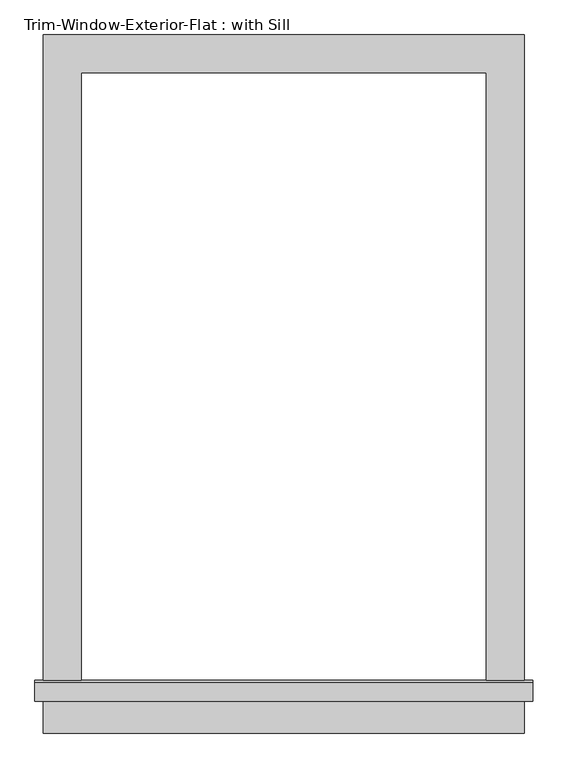
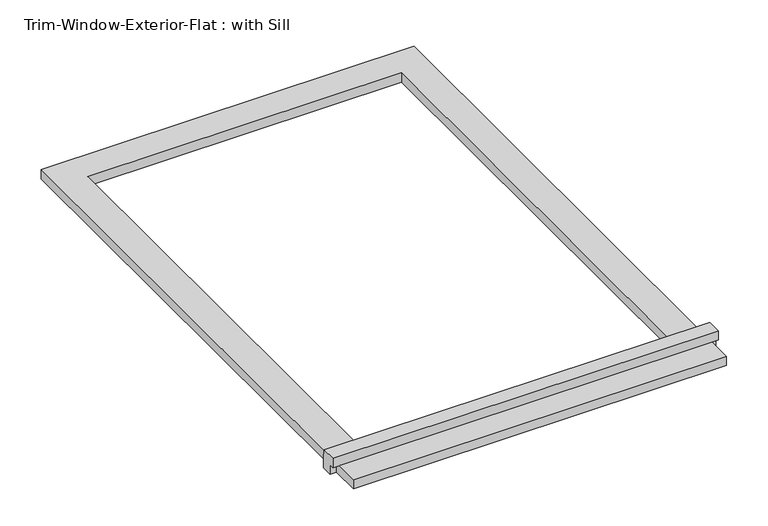
"""IFC4 building model written with IfcOpenShell, lengths in millimetres: proxy geometry, Trim-Window-Exterior-Flat : with Sill."""

from ifc_helpers import new_model, si_unit, frame, origin, origin_with_axes, place, context, project, spatial, polyline, outline, extrude, source, transform, mapped, element, save


def trim_window_exterior_flat_with_sill_a665a915(model_context):
    return source(origin(), model_context, "Body", "SweptSolid", [
        extrude(outline(polyline([(361.95, -936.5823709), (361.95, -993.7323709), (-361.95, -993.7323709), (-361.95, -936.5823709), (361.95, -936.5823709)])), origin_with_axes(), (0.0, 0.0, 1.0), 19.05),
        extrude(outline(polyline([(-946.15, 38.1), (-916.8580645, 38.1), (-914.4, 19.05), (-914.4, 0.0), (-936.5823709, 0.0), (-936.5823709, 19.05), (-946.15, 19.05), (-946.15, 38.1)])), frame((-374.65, 0.0, 0.0), z_axis=(1.0, 0.0, 0.0), x_axis=(0.0, 1.0, 0.0)), (0.0, 0.0, 1.0), 749.3),
        extrude(outline(polyline([(-361.95, 57.15), (361.95, 57.15), (361.95, -914.4), (304.8, -914.4), (304.8, 0.0), (-304.8, 0.0), (-304.8, -914.4), (-361.95, -914.4), (-361.95, 57.15)])), origin_with_axes(), (0.0, 0.0, 1.0), 19.05),
    ])


if __name__ == "__main__":
    model = new_model("IFC4")
    model_context = context("Model", 3, world=origin())
    ifc_project = project(units=[si_unit("LENGTHUNIT", "METRE", prefix="MILLI")], contexts=[model_context])
    site = spatial("IfcSite", under=ifc_project)
    building = spatial("IfcBuilding", under=site)
    placement = place(None, origin())
    trim_window_exterior_flat_with_sill_shape = trim_window_exterior_flat_with_sill_a665a915(model_context)
    element("IfcBuildingElementProxy", 1, Name="Trim-Window-Exterior-Flat : with Sill", ObjectType="Trim-Window-Exterior-Flat : with Sill", at=placement, inside=building, context=model_context, shape_type="MappedRepresentation", body=[
        mapped(trim_window_exterior_flat_with_sill_shape, transform((0.0, 0.0, 0.0), x_axis=(1.0, 0.0, 0.0), y_axis=(0.0, 1.0, 0.0), z_axis=(0.0, 0.0, 1.0))),
    ])
    save(model, "model.ifc")

# Revit data of these elements
# Type "Trim-Window-Exterior-Flat : with Sill"
#   Trim Width = 0' - 2 1/4"
#   Trim Thickness_Picture Frame = 0' - 1 1/4"
#   Trim Thickness_with Sill = 0' - 0 3/4"
#   Sill Thickness = 0' - 1 1/4"
#   Opening Width [instance default] = 2' - 0"
#   Opening Height [instance default] = 3' - 0"
#   Default Elevation = 4' - 0"
#   Sill = yes
#   Picture Frame = no
#   Trim Material [instance default] = none
# Element 1 (IfcBuildingElementProxy, "Trim-Window-Exterior-Flat : with Sill")
#   Trim Material = Clad - White
#   Materials on its faces: "Clad - White"
# Materials
#   "Clad - White": class "Wood", colour RGB 242 242 238, transparency 0, Cost = 0
